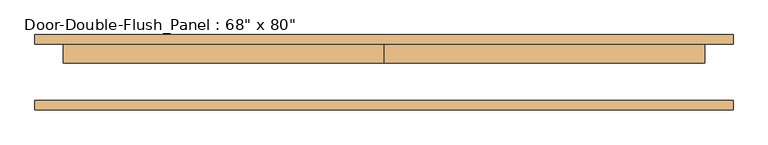
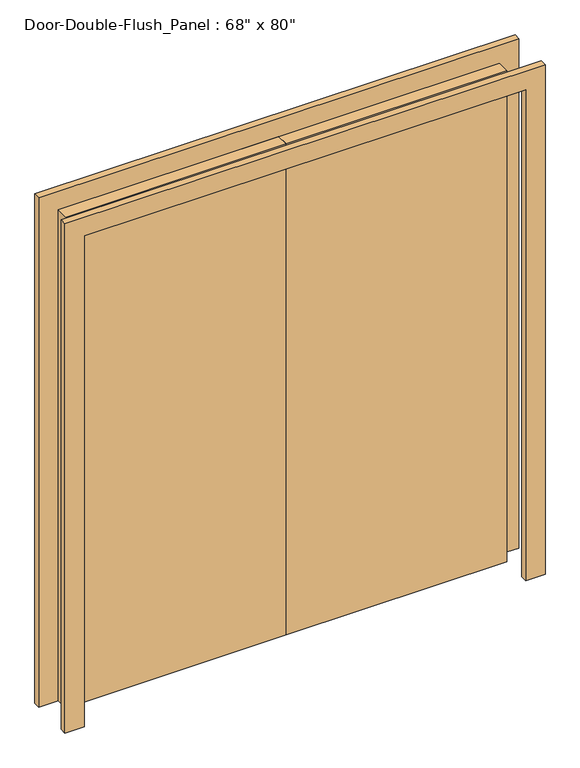
"""IFC4 building model written with IfcOpenShell, lengths in millimetres: door geometry."""

from ifc_helpers import new_model, si_unit, frame, origin, origin_with_axes, place, context, project, spatial, polyline, outline, extrude, source, transform, mapped, element, save


def door_74777eb6(model_context):
    return source(origin(), model_context, "Body", "SweptSolid", [
        extrude(outline(polyline([(2032.0, -863.6), (2032.0, 863.6), (0.0, 863.6), (0.0, 939.8), (2108.2, 939.8), (2108.2, -939.8), (0.0, -939.8), (0.0, -863.6), (2032.0, -863.6)])), frame((0.0, -101.6, 0.0), z_axis=(0.0, 1.0, 0.0), x_axis=(0.0, 0.0, 1.0)), (0.0, 0.0, 1.0), 25.4),
        extrude(outline(polyline([(2032.0, -863.6), (2032.0, 863.6), (0.0, 863.6), (0.0, 939.8), (2108.2, 939.8), (2108.2, -939.8), (0.0, -939.8), (0.0, -863.6), (2032.0, -863.6)])), frame((0.0, 76.2, 0.0), z_axis=(0.0, 1.0, 0.0), x_axis=(0.0, 0.0, 1.0)), (0.0, 0.0, 1.0), 25.4),
        extrude(outline(polyline([(0.0, 76.2), (863.6, 76.2), (863.6, 25.4), (0.0, 25.4), (0.0, 76.2)])), origin_with_axes(), (0.0, 0.0, 1.0), 2032.0),
        extrude(outline(polyline([(-863.6, 76.2), (0.0, 76.2), (0.0, 25.4), (-863.6, 25.4), (-863.6, 76.2)])), origin_with_axes(), (0.0, 0.0, 1.0), 2032.0),
    ])


if __name__ == "__main__":
    model = new_model("IFC4")
    model_context = context("Model", 3, world=origin())
    ifc_project = project(units=[si_unit("LENGTHUNIT", "METRE", prefix="MILLI")], contexts=[model_context])
    site = spatial("IfcSite", under=ifc_project)
    building = spatial("IfcBuilding", under=site)
    placement = place(None, origin())
    door_shape = door_74777eb6(model_context)
    element("IfcDoor", 1, ObjectType="Door-Double-Flush_Panel : 68\" x 80\"", at=placement, inside=building, context=model_context, shape_type="MappedRepresentation", body=[
        mapped(door_shape, transform((0.0, 0.0, 0.0), x_axis=(1.0, 0.0, 0.0), y_axis=(0.0, 1.0, 0.0), z_axis=(0.0, 0.0, 1.0))),
    ])
    save(model, "model.ifc")

# Revit data of these elements
# Type "Door-Double-Flush_Panel : 68\" x 80\""
#   Type Mark = "8"
#   Construction Type Id = "DOOR"
#   Assembly Code = "C1020"
#   Analytic Construction = "Wooden"
#   Thickness = 0' - 2"
#   Thermal Resistance (R) = 2.5876 (h·ft²·°F)/BTU
#   Swing Angle [instance default] = 90.00°
#   Panel Width = 2' - 10"
#   Heat Transfer Coefficient (U) = 0.3865 BTU/(h·ft²·°F)
#   Height = 6' - 8"
#   Trim Projection Ext = 0' - 1"
#   Trim Projection Int = 0' - 1"
#   Trim Width = 0' - 3"
#   Width = 5' - 8"
#   Define Thermal Properties by = 1
#   Panel Material = Wood - Birch - Solid Stained Light Low Gloss
#   Trim Material = Paint - Sienna
#   Visual Light Transmittance = 0
#   Solar Heat Gain Coefficient = 0
#   Function = (empty or 0)
#   Wall Closure = (empty or 0)
# Element 1 (IfcDoor, "Door-Double-Flush_Panel : 68\" x 80\"")
#   Materials on its faces: "Paint - Sienna", "Wood - Birch - Solid Stained Light Low Gloss"
# Materials
#   "Wood - Birch - Solid Stained Light Low Gloss": class "Wood", colour RGB 210 159 95, transparency 0, Cost = 0
#   "Paint - Sienna": colour RGB 118 70 51, transparency 0, Cost = 0
